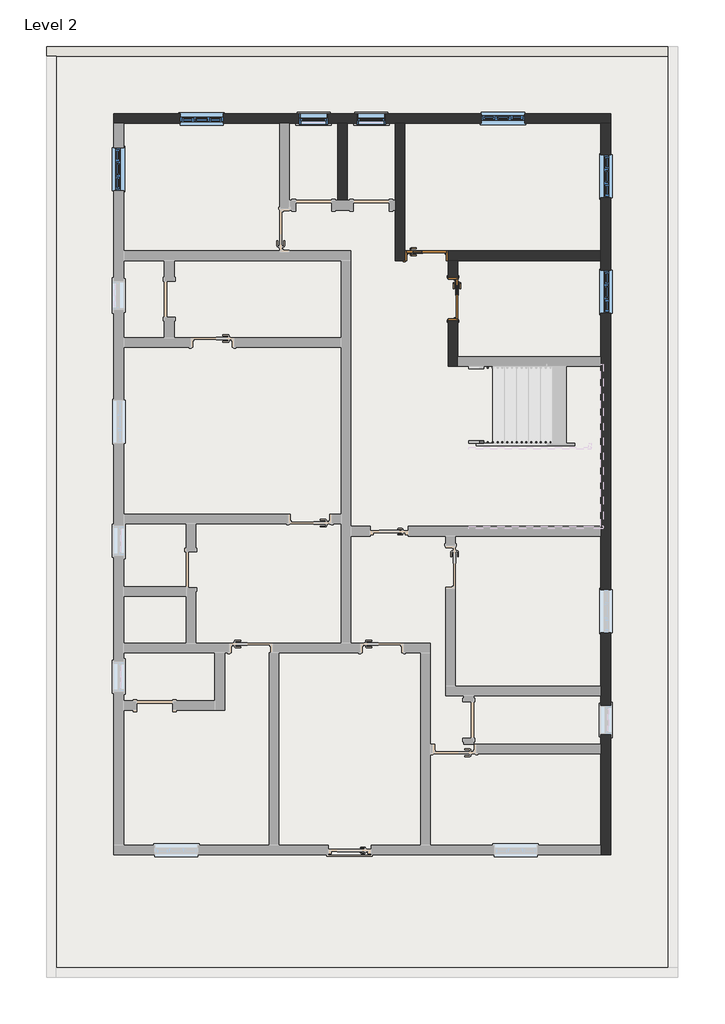
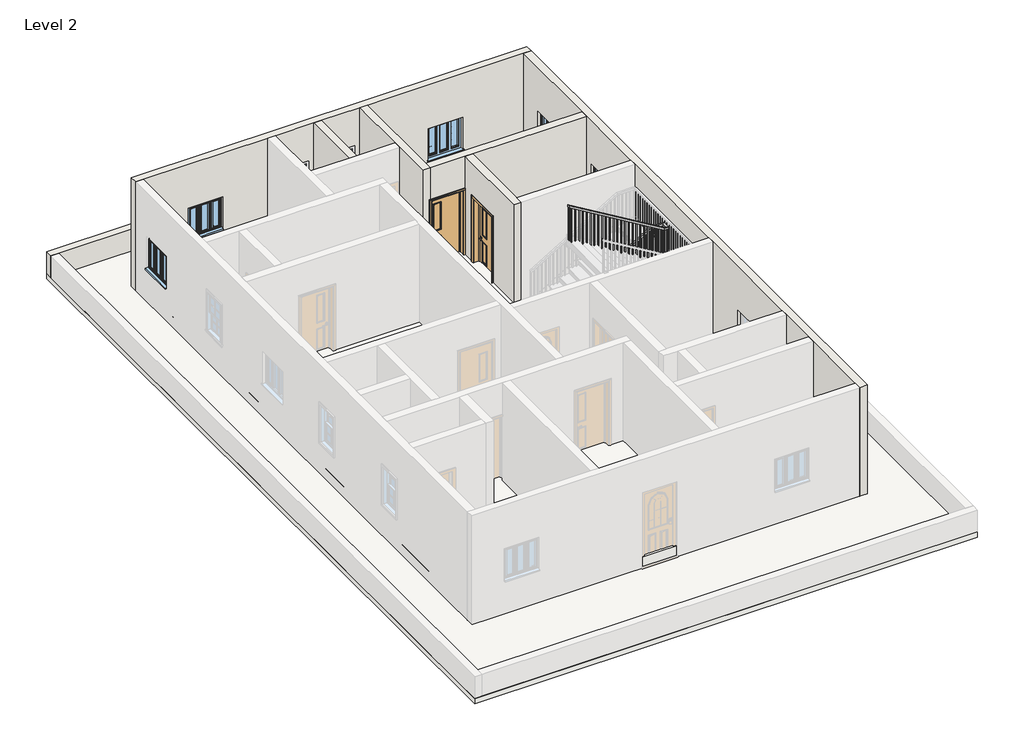
# One storey, part 2 of 3: 7 walls, 7 windows, 2 doors, 2 slabs, 1 railing, 1 roof.
"""IFC4 building model written with IfcOpenShell, lengths in millimetres."""

from ifc_helpers import new_model, si_unit, frame, origin, place, context, project, spatial, polyline, outline, extrude, faceted_brep, transform, mapped, element, save
from components import door_aa1d4bf3, window_679d2811, windows_tpl_w_glazing_bars_910x910mm_9d987a72

model = new_model("IFC4")

# Units and contexts
model_context = context("Model", 3, world=origin())
ifc_project = project(units=[si_unit("LENGTHUNIT", "METRE", prefix="MILLI")], contexts=[model_context])

# Site, building, storey
site = spatial("IfcSite", under=ifc_project)
building = spatial("IfcBuilding", under=site)
storey = spatial("IfcBuildingStorey", under=building, Name="Level 2", Elevation=3048.0)

# Doors
placement = place(None, origin())
door_shape = door_aa1d4bf3(model_context)
element("IfcDoor", 1, ObjectType="Doors_IntSgl_3 : 7'-3\"", at=placement, inside=storey, context=model_context, shape_type="MappedRepresentation", body=[
    mapped(door_shape, transform((-7303.1711241, 14069.3344295, 3048.0), x_axis=(1.0, 0.0, 0.0), y_axis=(0.0, 1.0, 0.0), z_axis=(0.0, 0.0, 1.0))),
])
element("IfcDoor", 2, ObjectType="Doors_IntSgl_3 : 7'-3\"", at=placement, inside=storey, context=model_context, shape_type="MappedRepresentation", body=[
    mapped(door_shape, transform((-6744.3711241, 13154.9344295, 3048.0), x_axis=(0.0, -1.0, 0.0), y_axis=(1.0, 0.0, 0.0), z_axis=(0.0, 0.0, 1.0))),
])

# Railing
element("IfcRailing", 3, ObjectType="Handrail - Rectangular", at=placement, inside=storey, context=model_context, shape_type="SolidModel", body=[
    faceted_brep([(-6414.1711241, 10157.7344295, 4114.8), (-6414.1711241, 10157.7344295, 4055.5575287), (-6414.1711241, 10106.9344295, 4055.5575287), (-6414.1711241, 10106.9344295, 4114.8), (-4128.1711241, 10157.7344295, 5486.4), (-4114.1003386, 10157.7344295, 5435.6), (-4114.1003386, 10106.9344295, 5435.6), (-4128.1711241, 10106.9344295, 5486.4), (-3772.5711241, 10157.7344295, 5486.4), (-3772.5711241, 10157.7344295, 5435.6), (-3823.3711241, 10106.9344295, 5435.6), (-3823.3711241, 10106.9344295, 5486.4), (-3772.5711241, 9929.1344295, 5486.4), (-3772.5711241, 9929.1344295, 5435.6), (-3823.3711241, 9979.9344295, 5435.6), (-3823.3711241, 9979.9344295, 5486.4), (-3874.1711241, 9929.1344295, 5486.4), (-3888.2419095, 9929.1344295, 5435.6), (-3888.2419095, 9979.9344295, 5435.6), (-3874.1711241, 9979.9344295, 5486.4), (-6414.1711241, 9929.1344295, 7010.4), (-6414.1711241, 9979.9344295, 7010.4), (-6414.1711241, 9979.9344295, 6951.1575287), (-6414.1711241, 9929.1344295, 6951.1575287)], [[[0, 1, 2, 3]], [[1, 0, 4, 5]], [[2, 1, 5, 6]], [[3, 2, 6, 7]], [[0, 3, 7, 4]], [[5, 4, 8, 9]], [[6, 5, 9, 10]], [[7, 6, 10, 11]], [[4, 7, 11, 8]], [[9, 8, 12, 13]], [[10, 9, 13, 14]], [[11, 10, 14, 15]], [[8, 11, 15, 12]], [[13, 12, 16, 17]], [[14, 13, 17, 18]], [[15, 14, 18, 19]], [[12, 15, 19, 16]], [[20, 21, 22, 23]], [[17, 16, 20, 23]], [[18, 17, 23, 22]], [[19, 18, 22, 21]], [[16, 19, 21, 20]]]),
    extrude(outline(polyline([(6899.7225287, -6328.4461241), (6911.1525287, -6347.4961241), (5943.6, -6347.4961241), (5943.6, -6328.4461241), (6899.7225287, -6328.4461241)])), frame((0.0, 9945.0094295, 0.0), z_axis=(0.0, 1.0, 0.0), x_axis=(0.0, 0.0, 1.0)), (0.0, 0.0, 1.0), 19.05),
    extrude(outline(polyline([(6838.7625287, -6226.8461241), (6850.1925287, -6245.8961241), (5943.6, -6245.8961241), (5943.6, -6226.8461241), (6838.7625287, -6226.8461241)])), frame((0.0, 9945.0094295, 0.0), z_axis=(0.0, 1.0, 0.0), x_axis=(0.0, 0.0, 1.0)), (0.0, 0.0, 1.0), 19.05),
    extrude(outline(polyline([(6777.8025287, -6125.2461241), (6789.2325287, -6144.2961241), (5791.2, -6144.2961241), (5791.2, -6125.2461241), (6777.8025287, -6125.2461241)])), frame((0.0, 9945.0094295, 0.0), z_axis=(0.0, 1.0, 0.0), x_axis=(0.0, 0.0, 1.0)), (0.0, 0.0, 1.0), 19.05),
    extrude(outline(polyline([(6716.8425287, -6023.6461241), (6728.2725287, -6042.6961241), (5791.2, -6042.6961241), (5791.2, -6023.6461241), (6716.8425287, -6023.6461241)])), frame((0.0, 9945.0094295, 0.0), z_axis=(0.0, 1.0, 0.0), x_axis=(0.0, 0.0, 1.0)), (0.0, 0.0, 1.0), 19.05),
    extrude(outline(polyline([(6655.8825287, -5922.0461241), (6667.3125287, -5941.0961241), (5791.2, -5941.0961241), (5791.2, -5922.0461241), (6655.8825287, -5922.0461241)])), frame((0.0, 9945.0094295, 0.0), z_axis=(0.0, 1.0, 0.0), x_axis=(0.0, 0.0, 1.0)), (0.0, 0.0, 1.0), 19.05),
    extrude(outline(polyline([(6594.9225287, -5820.4461241), (6606.3525287, -5839.4961241), (5638.8, -5839.4961241), (5638.8, -5820.4461241), (6594.9225287, -5820.4461241)])), frame((0.0, 9945.0094295, 0.0), z_axis=(0.0, 1.0, 0.0), x_axis=(0.0, 0.0, 1.0)), (0.0, 0.0, 1.0), 19.05),
    extrude(outline(polyline([(6533.9625287, -5718.8461241), (6545.3925287, -5737.8961241), (5638.8, -5737.8961241), (5638.8, -5718.8461241), (6533.9625287, -5718.8461241)])), frame((0.0, 9945.0094295, 0.0), z_axis=(0.0, 1.0, 0.0), x_axis=(0.0, 0.0, 1.0)), (0.0, 0.0, 1.0), 19.05),
    extrude(outline(polyline([(6473.0025287, -5617.2461241), (6484.4325287, -5636.2961241), (5486.4, -5636.2961241), (5486.4, -5617.2461241), (6473.0025287, -5617.2461241)])), frame((0.0, 9945.0094295, 0.0), z_axis=(0.0, 1.0, 0.0), x_axis=(0.0, 0.0, 1.0)), (0.0, 0.0, 1.0), 19.05),
    extrude(outline(polyline([(6412.0425287, -5515.6461241), (6423.4725287, -5534.6961241), (5486.4, -5534.6961241), (5486.4, -5515.6461241), (6412.0425287, -5515.6461241)])), frame((0.0, 9945.0094295, 0.0), z_axis=(0.0, 1.0, 0.0), x_axis=(0.0, 0.0, 1.0)), (0.0, 0.0, 1.0), 19.05),
    extrude(outline(polyline([(6351.0825287, -5414.0461241), (6362.5125287, -5433.0961241), (5486.4, -5433.0961241), (5486.4, -5414.0461241), (6351.0825287, -5414.0461241)])), frame((0.0, 9945.0094295, 0.0), z_axis=(0.0, 1.0, 0.0), x_axis=(0.0, 0.0, 1.0)), (0.0, 0.0, 1.0), 19.05),
    extrude(outline(polyline([(6290.1225287, -5312.4461241), (6301.5525287, -5331.4961241), (5334.0, -5331.4961241), (5334.0, -5312.4461241), (6290.1225287, -5312.4461241)])), frame((0.0, 9945.0094295, 0.0), z_axis=(0.0, 1.0, 0.0), x_axis=(0.0, 0.0, 1.0)), (0.0, 0.0, 1.0), 19.05),
    extrude(outline(polyline([(6229.1625287, -5210.8461241), (6240.5925287, -5229.8961241), (5334.0, -5229.8961241), (5334.0, -5210.8461241), (6229.1625287, -5210.8461241)])), frame((0.0, 9945.0094295, 0.0), z_axis=(0.0, 1.0, 0.0), x_axis=(0.0, 0.0, 1.0)), (0.0, 0.0, 1.0), 19.05),
    extrude(outline(polyline([(6168.2025287, -5109.2461241), (6179.6325287, -5128.2961241), (5181.6, -5128.2961241), (5181.6, -5109.2461241), (6168.2025287, -5109.2461241)])), frame((0.0, 9945.0094295, 0.0), z_axis=(0.0, 1.0, 0.0), x_axis=(0.0, 0.0, 1.0)), (0.0, 0.0, 1.0), 19.05),
    extrude(outline(polyline([(6107.2425287, -5007.6461241), (6118.6725287, -5026.6961241), (5181.6, -5026.6961241), (5181.6, -5007.6461241), (6107.2425287, -5007.6461241)])), frame((0.0, 9945.0094295, 0.0), z_axis=(0.0, 1.0, 0.0), x_axis=(0.0, 0.0, 1.0)), (0.0, 0.0, 1.0), 19.05),
    extrude(outline(polyline([(6046.2825287, -4906.0461241), (6057.7125287, -4925.0961241), (5181.6, -4925.0961241), (5181.6, -4906.0461241), (6046.2825287, -4906.0461241)])), frame((0.0, 9945.0094295, 0.0), z_axis=(0.0, 1.0, 0.0), x_axis=(0.0, 0.0, 1.0)), (0.0, 0.0, 1.0), 19.05),
    extrude(outline(polyline([(5985.3225287, -4804.4461241), (5996.7525287, -4823.4961241), (5029.2, -4823.4961241), (5029.2, -4804.4461241), (5985.3225287, -4804.4461241)])), frame((0.0, 9945.0094295, 0.0), z_axis=(0.0, 1.0, 0.0), x_axis=(0.0, 0.0, 1.0)), (0.0, 0.0, 1.0), 19.05),
    extrude(outline(polyline([(5924.3625287, -4702.8461241), (5935.7925287, -4721.8961241), (5029.2, -4721.8961241), (5029.2, -4702.8461241), (5924.3625287, -4702.8461241)])), frame((0.0, 9945.0094295, 0.0), z_axis=(0.0, 1.0, 0.0), x_axis=(0.0, 0.0, 1.0)), (0.0, 0.0, 1.0), 19.05),
    extrude(outline(polyline([(5863.4025287, -4601.2461241), (5874.8325287, -4620.2961241), (4876.8, -4620.2961241), (4876.8, -4601.2461241), (5863.4025287, -4601.2461241)])), frame((0.0, 9945.0094295, 0.0), z_axis=(0.0, 1.0, 0.0), x_axis=(0.0, 0.0, 1.0)), (0.0, 0.0, 1.0), 19.05),
    extrude(outline(polyline([(5802.4425287, -4499.6461241), (5813.8725287, -4518.6961241), (4876.8, -4518.6961241), (4876.8, -4499.6461241), (5802.4425287, -4499.6461241)])), frame((0.0, 9945.0094295, 0.0), z_axis=(0.0, 1.0, 0.0), x_axis=(0.0, 0.0, 1.0)), (0.0, 0.0, 1.0), 19.05),
    extrude(outline(polyline([(5741.4825287, -4398.0461241), (5752.9125287, -4417.0961241), (4876.8, -4417.0961241), (4876.8, -4398.0461241), (5741.4825287, -4398.0461241)])), frame((0.0, 9945.0094295, 0.0), z_axis=(0.0, 1.0, 0.0), x_axis=(0.0, 0.0, 1.0)), (0.0, 0.0, 1.0), 19.05),
    extrude(outline(polyline([(5680.5225287, -4296.4461241), (5691.9525287, -4315.4961241), (4724.4, -4315.4961241), (4724.4, -4296.4461241), (5680.5225287, -4296.4461241)])), frame((0.0, 9945.0094295, 0.0), z_axis=(0.0, 1.0, 0.0), x_axis=(0.0, 0.0, 1.0)), (0.0, 0.0, 1.0), 19.05),
    extrude(outline(polyline([(5619.5625287, -4194.8461241), (5630.9925287, -4213.8961241), (4724.4, -4213.8961241), (4724.4, -4194.8461241), (5619.5625287, -4194.8461241)])), frame((0.0, 9945.0094295, 0.0), z_axis=(0.0, 1.0, 0.0), x_axis=(0.0, 0.0, 1.0)), (0.0, 0.0, 1.0), 19.05),
    extrude(outline(polyline([(5558.6025287, -4093.2461241), (5570.0325287, -4112.2961241), (4572.0, -4112.2961241), (4572.0, -4093.2461241), (5558.6025287, -4093.2461241)])), frame((0.0, 9945.0094295, 0.0), z_axis=(0.0, 1.0, 0.0), x_axis=(0.0, 0.0, 1.0)), (0.0, 0.0, 1.0), 19.05),
    extrude(outline(polyline([(5497.6425287, -3991.6461241), (5509.0725287, -4010.6961241), (4572.0, -4010.6961241), (4572.0, -3991.6461241), (5497.6425287, -3991.6461241)])), frame((0.0, 9945.0094295, 0.0), z_axis=(0.0, 1.0, 0.0), x_axis=(0.0, 0.0, 1.0)), (0.0, 0.0, 1.0), 19.05),
    extrude(outline(polyline([(5436.6825287, -3890.0461241), (5448.1125287, -3909.0961241), (4572.0, -3909.0961241), (4572.0, -3890.0461241), (5436.6825287, -3890.0461241)])), frame((0.0, 9945.0094295, 0.0), z_axis=(0.0, 1.0, 0.0), x_axis=(0.0, 0.0, 1.0)), (0.0, 0.0, 1.0), 19.05),
    extrude(outline(polyline([(-3807.4961241, 10040.2594295), (-3788.4461241, 10040.2594295), (-3788.4461241, 10021.2094295), (-3807.4961241, 10021.2094295), (-3807.4961241, 10040.2594295)])), frame((0.0, 0.0, 4572.0), z_axis=(0.0, 0.0, 1.0), x_axis=(1.0, 0.0, 0.0)), (0.0, 0.0, 1.0), 863.6),
    extrude(outline(polyline([(-3883.6961241, 10122.8094295), (-3883.6961241, 10141.8594295), (-3864.6461241, 10141.8594295), (-3864.6461241, 10122.8094295), (-3883.6961241, 10122.8094295)])), frame((0.0, 0.0, 4572.0), z_axis=(0.0, 0.0, 1.0), x_axis=(1.0, 0.0, 0.0)), (0.0, 0.0, 1.0), 863.6),
    extrude(outline(polyline([(-3985.2961241, 10122.8094295), (-3985.2961241, 10141.8594295), (-3966.2461241, 10141.8594295), (-3966.2461241, 10122.8094295), (-3985.2961241, 10122.8094295)])), frame((0.0, 0.0, 4572.0), z_axis=(0.0, 0.0, 1.0), x_axis=(1.0, 0.0, 0.0)), (0.0, 0.0, 1.0), 863.6),
    extrude(outline(polyline([(-4086.8961241, 10122.8094295), (-4086.8961241, 10141.8594295), (-4067.8461241, 10141.8594295), (-4067.8461241, 10122.8094295), (-4086.8961241, 10122.8094295)])), frame((0.0, 0.0, 4572.0), z_axis=(0.0, 0.0, 1.0), x_axis=(1.0, 0.0, 0.0)), (0.0, 0.0, 1.0), 863.6),
    extrude(outline(polyline([(5402.3925287, -4169.4461241), (5390.9625287, -4188.4961241), (4419.6, -4188.4961241), (4419.6, -4169.4461241), (5402.3925287, -4169.4461241)])), frame((0.0, 10122.8094295, 0.0), z_axis=(0.0, 1.0, 0.0), x_axis=(0.0, 0.0, 1.0)), (0.0, 0.0, 1.0), 19.05),
    extrude(outline(polyline([(5341.4325287, -4271.0461241), (5330.0025287, -4290.0961241), (4419.6, -4290.0961241), (4419.6, -4271.0461241), (5341.4325287, -4271.0461241)])), frame((0.0, 10122.8094295, 0.0), z_axis=(0.0, 1.0, 0.0), x_axis=(0.0, 0.0, 1.0)), (0.0, 0.0, 1.0), 19.05),
    extrude(outline(polyline([(5280.4725287, -4372.6461241), (5269.0425287, -4391.6961241), (4419.6, -4391.6961241), (4419.6, -4372.6461241), (5280.4725287, -4372.6461241)])), frame((0.0, 10122.8094295, 0.0), z_axis=(0.0, 1.0, 0.0), x_axis=(0.0, 0.0, 1.0)), (0.0, 0.0, 1.0), 19.05),
    extrude(outline(polyline([(5219.5125287, -4474.2461241), (5208.0825287, -4493.2961241), (4267.2, -4493.2961241), (4267.2, -4474.2461241), (5219.5125287, -4474.2461241)])), frame((0.0, 10122.8094295, 0.0), z_axis=(0.0, 1.0, 0.0), x_axis=(0.0, 0.0, 1.0)), (0.0, 0.0, 1.0), 19.05),
    extrude(outline(polyline([(5158.5525287, -4575.8461241), (5147.1225287, -4594.8961241), (4267.2, -4594.8961241), (4267.2, -4575.8461241), (5158.5525287, -4575.8461241)])), frame((0.0, 10122.8094295, 0.0), z_axis=(0.0, 1.0, 0.0), x_axis=(0.0, 0.0, 1.0)), (0.0, 0.0, 1.0), 19.05),
    extrude(outline(polyline([(5097.5925287, -4677.4461241), (5086.1625287, -4696.4961241), (4114.8, -4696.4961241), (4114.8, -4677.4461241), (5097.5925287, -4677.4461241)])), frame((0.0, 10122.8094295, 0.0), z_axis=(0.0, 1.0, 0.0), x_axis=(0.0, 0.0, 1.0)), (0.0, 0.0, 1.0), 19.05),
    extrude(outline(polyline([(5036.6325287, -4779.0461241), (5025.2025287, -4798.0961241), (4114.8, -4798.0961241), (4114.8, -4779.0461241), (5036.6325287, -4779.0461241)])), frame((0.0, 10122.8094295, 0.0), z_axis=(0.0, 1.0, 0.0), x_axis=(0.0, 0.0, 1.0)), (0.0, 0.0, 1.0), 19.05),
    extrude(outline(polyline([(4975.6725287, -4880.6461241), (4964.2425287, -4899.6961241), (4114.8, -4899.6961241), (4114.8, -4880.6461241), (4975.6725287, -4880.6461241)])), frame((0.0, 10122.8094295, 0.0), z_axis=(0.0, 1.0, 0.0), x_axis=(0.0, 0.0, 1.0)), (0.0, 0.0, 1.0), 19.05),
    extrude(outline(polyline([(4914.7125287, -4982.2461241), (4903.2825287, -5001.2961241), (3962.4, -5001.2961241), (3962.4, -4982.2461241), (4914.7125287, -4982.2461241)])), frame((0.0, 10122.8094295, 0.0), z_axis=(0.0, 1.0, 0.0), x_axis=(0.0, 0.0, 1.0)), (0.0, 0.0, 1.0), 19.05),
    extrude(outline(polyline([(4853.7525287, -5083.8461241), (4842.3225287, -5102.8961241), (3962.4, -5102.8961241), (3962.4, -5083.8461241), (4853.7525287, -5083.8461241)])), frame((0.0, 10122.8094295, 0.0), z_axis=(0.0, 1.0, 0.0), x_axis=(0.0, 0.0, 1.0)), (0.0, 0.0, 1.0), 19.05),
    extrude(outline(polyline([(4792.7925287, -5185.4461241), (4781.3625287, -5204.4961241), (3810.0, -5204.4961241), (3810.0, -5185.4461241), (4792.7925287, -5185.4461241)])), frame((0.0, 10122.8094295, 0.0), z_axis=(0.0, 1.0, 0.0), x_axis=(0.0, 0.0, 1.0)), (0.0, 0.0, 1.0), 19.05),
    extrude(outline(polyline([(4731.8325287, -5287.0461241), (4720.4025287, -5306.0961241), (3810.0, -5306.0961241), (3810.0, -5287.0461241), (4731.8325287, -5287.0461241)])), frame((0.0, 10122.8094295, 0.0), z_axis=(0.0, 1.0, 0.0), x_axis=(0.0, 0.0, 1.0)), (0.0, 0.0, 1.0), 19.05),
    extrude(outline(polyline([(4670.8725287, -5388.6461241), (4659.4425287, -5407.6961241), (3810.0, -5407.6961241), (3810.0, -5388.6461241), (4670.8725287, -5388.6461241)])), frame((0.0, 10122.8094295, 0.0), z_axis=(0.0, 1.0, 0.0), x_axis=(0.0, 0.0, 1.0)), (0.0, 0.0, 1.0), 19.05),
    extrude(outline(polyline([(4609.9125287, -5490.2461241), (4598.4825287, -5509.2961241), (3657.6, -5509.2961241), (3657.6, -5490.2461241), (4609.9125287, -5490.2461241)])), frame((0.0, 10122.8094295, 0.0), z_axis=(0.0, 1.0, 0.0), x_axis=(0.0, 0.0, 1.0)), (0.0, 0.0, 1.0), 19.05),
    extrude(outline(polyline([(4548.9525287, -5591.8461241), (4537.5225287, -5610.8961241), (3657.6, -5610.8961241), (3657.6, -5591.8461241), (4548.9525287, -5591.8461241)])), frame((0.0, 10122.8094295, 0.0), z_axis=(0.0, 1.0, 0.0), x_axis=(0.0, 0.0, 1.0)), (0.0, 0.0, 1.0), 19.05),
    extrude(outline(polyline([(4487.9925287, -5693.4461241), (4476.5625287, -5712.4961241), (3505.2, -5712.4961241), (3505.2, -5693.4461241), (4487.9925287, -5693.4461241)])), frame((0.0, 10122.8094295, 0.0), z_axis=(0.0, 1.0, 0.0), x_axis=(0.0, 0.0, 1.0)), (0.0, 0.0, 1.0), 19.05),
    extrude(outline(polyline([(4427.0325287, -5795.0461241), (4415.6025287, -5814.0961241), (3505.2, -5814.0961241), (3505.2, -5795.0461241), (4427.0325287, -5795.0461241)])), frame((0.0, 10122.8094295, 0.0), z_axis=(0.0, 1.0, 0.0), x_axis=(0.0, 0.0, 1.0)), (0.0, 0.0, 1.0), 19.05),
    extrude(outline(polyline([(4366.0725287, -5896.6461241), (4354.6425287, -5915.6961241), (3505.2, -5915.6961241), (3505.2, -5896.6461241), (4366.0725287, -5896.6461241)])), frame((0.0, 10122.8094295, 0.0), z_axis=(0.0, 1.0, 0.0), x_axis=(0.0, 0.0, 1.0)), (0.0, 0.0, 1.0), 19.05),
    extrude(outline(polyline([(4305.1125287, -5998.2461241), (4293.6825287, -6017.2961241), (3352.8, -6017.2961241), (3352.8, -5998.2461241), (4305.1125287, -5998.2461241)])), frame((0.0, 10122.8094295, 0.0), z_axis=(0.0, 1.0, 0.0), x_axis=(0.0, 0.0, 1.0)), (0.0, 0.0, 1.0), 19.05),
    extrude(outline(polyline([(4244.1525287, -6099.8461241), (4232.7225287, -6118.8961241), (3352.8, -6118.8961241), (3352.8, -6099.8461241), (4244.1525287, -6099.8461241)])), frame((0.0, 10122.8094295, 0.0), z_axis=(0.0, 1.0, 0.0), x_axis=(0.0, 0.0, 1.0)), (0.0, 0.0, 1.0), 19.05),
    extrude(outline(polyline([(4183.1925287, -6201.4461241), (4171.7625287, -6220.4961241), (3200.4, -6220.4961241), (3200.4, -6201.4461241), (4183.1925287, -6201.4461241)])), frame((0.0, 10122.8094295, 0.0), z_axis=(0.0, 1.0, 0.0), x_axis=(0.0, 0.0, 1.0)), (0.0, 0.0, 1.0), 19.05),
    extrude(outline(polyline([(4122.2325287, -6303.0461241), (4110.8025287, -6322.0961241), (3200.4, -6322.0961241), (3200.4, -6303.0461241), (4122.2325287, -6303.0461241)])), frame((0.0, 10122.8094295, 0.0), z_axis=(0.0, 1.0, 0.0), x_axis=(0.0, 0.0, 1.0)), (0.0, 0.0, 1.0), 19.05),
    extrude(outline(polyline([(-3807.4961241, 9964.0594295), (-3788.4461241, 9964.0594295), (-3788.4461241, 9945.0094295), (-3807.4961241, 9945.0094295), (-3807.4961241, 9964.0594295)])), frame((0.0, 0.0, 4572.0), z_axis=(0.0, 0.0, 1.0), x_axis=(1.0, 0.0, 0.0)), (0.0, 0.0, 1.0), 863.6),
    extrude(outline(polyline([(-3807.4961241, 10122.8094295), (-3807.4961241, 10141.8594295), (-3788.4461241, 10141.8594295), (-3788.4461241, 10122.8094295), (-3807.4961241, 10122.8094295)])), frame((0.0, 0.0, 4572.0), z_axis=(0.0, 0.0, 1.0), x_axis=(1.0, 0.0, 0.0)), (0.0, 0.0, 1.0), 863.6),
    extrude(outline(polyline([(6939.7275287, -6395.1211241), (6951.1575287, -6414.1711241), (5943.6, -6414.1711241), (5943.6, -6395.1211241), (6939.7275287, -6395.1211241)])), frame((0.0, 9945.0094295, 0.0), z_axis=(0.0, 1.0, 0.0), x_axis=(0.0, 0.0, 1.0)), (0.0, 0.0, 1.0), 19.05),
    extrude(outline(polyline([(4066.9875287, -6395.1211241), (4055.5575287, -6414.1711241), (3200.4, -6414.1711241), (3200.4, -6395.1211241), (4066.9875287, -6395.1211241)])), frame((0.0, 10122.8094295, 0.0), z_axis=(0.0, 1.0, 0.0), x_axis=(0.0, 0.0, 1.0)), (0.0, 0.0, 1.0), 19.05),
])

# Roof
element("IfcRoof", 4, ObjectType="Generic - 12\"", at=placement, inside=storey, context=model_context, shape_type="SweptSolid", body=[
    extrude(outline(polyline([(-13907.1711241, 17066.5344295), (-3416.9711241, 17066.5344295), (-3416.9711241, 1420.1344295), (-13907.1711241, 1420.1344295), (-13907.1711241, 17066.5344295)])), frame((0.0, 0.0, 3048.0), z_axis=(0.0, 0.0, 1.0), x_axis=(1.0, 0.0, 0.0)), (0.0, 0.0, 1.0), 304.8),
])

# Slabs
element("IfcSlab", 5, ObjectType="Generic - 12\" 2", at=placement, inside=storey, context=model_context, shape_type="SweptSolid", body=[
    extrude(outline(polyline([(-3416.9711241, 17066.5344295), (-3416.9711241, 1420.1344295), (-13907.1711241, 1420.1344295), (-13907.1711241, 17066.5344295), (-3416.9711241, 17066.5344295)])), frame((0.0, 0.0, 2895.6), z_axis=(0.0, 0.0, 1.0), x_axis=(1.0, 0.0, 0.0)), (0.0, 0.0, 1.0), 152.4),
])
element("IfcSlab", 6, ObjectType="Generic - 12\" 3", at=placement, inside=storey, context=model_context, shape_type="SweptSolid", body=[
    extrude(outline(polyline([(-1994.5711241, 18488.2009778), (-1994.5711241, -1171.3990222), (-15329.5711241, -1171.3990222), (-15329.5711241, 18488.2009778), (-1994.5711241, 18488.2009778)])), frame((0.0, 0.0, 2895.6), z_axis=(0.0, 0.0, 1.0), x_axis=(1.0, 0.0, 0.0)), (0.0, 0.0, 1.0), 152.4),
])

# Walls
element("IfcWall", 7, ObjectType="Generic -4.5\" p", at=placement, inside=storey, context=model_context, shape_type="SweptSolid", body=[
    extrude(outline(polyline([(-9182.7711241, 15237.7344295), (-9182.7711241, 16863.3344295), (-8979.5711241, 16863.3344295), (-8979.5711241, 15237.7344295), (-9182.7711241, 15237.7344295)])), frame((0.0, 0.0, 3048.0), z_axis=(0.0, 0.0, 1.0), x_axis=(1.0, 0.0, 0.0)), (0.0, 0.0, 1.0), 3048.0),
])
element("IfcWall", 8, ObjectType="Generic -4.5\" p", at=placement, inside=storey, context=model_context, shape_type="Brep", body=[
    faceted_brep([(-7963.5711241, 16863.3344295, 3048.0), (-7963.5711241, 15237.7344295, 3048.0), (-7963.5711241, 15034.5344295, 3048.0), (-7963.5711241, 13967.7344295, 3048.0), (-7963.5711241, 13967.7344295, 6096.0), (-7963.5711241, 15034.5344295, 6096.0), (-7963.5711241, 15237.7344295, 6096.0), (-7963.5711241, 16863.3344295, 6096.0), (-7760.3711241, 16863.3344295, 3048.0), (-7760.3711241, 16863.3344295, 6096.0), (-7760.3711241, 14170.9344295, 6096.0), (-7760.3711241, 13967.7344295, 6096.0), (-7760.3711241, 13967.7344295, 5181.6), (-7760.3711241, 13967.7344295, 3048.0)], [[[0, 1, 2, 3, 4, 5, 6, 7]], [[8, 9, 10, 11, 12, 13]], [[3, 2, 1, 0, 8, 13]], [[7, 6, 5, 4, 11, 10, 9]], [[0, 7, 9, 8]], [[4, 3, 13, 12, 11]]]),
])
element("IfcWall", 9, ObjectType="Generic -4.5\" p", at=placement, inside=storey, context=model_context, shape_type="Brep", body=[
    faceted_brep([(-7760.3711241, 14170.9344295, 6096.0), (-3620.1711241, 14170.9344295, 6096.0), (-3620.1711241, 14170.9344295, 3048.0), (-6845.9711241, 14170.9344295, 3048.0), (-6845.9711241, 14170.9344295, 5181.6), (-7760.3711241, 14170.9344295, 5181.6), (-3620.1711241, 13967.7344295, 6096.0), (-6642.7711241, 13967.7344295, 6096.0), (-6845.9711241, 13967.7344295, 6096.0), (-7760.3711241, 13967.7344295, 6096.0), (-7760.3711241, 13967.7344295, 5181.6), (-6845.9711241, 13967.7344295, 5181.6), (-6845.9711241, 13967.7344295, 3048.0), (-6642.7711241, 13967.7344295, 3048.0), (-3620.1711241, 13967.7344295, 3048.0)], [[[0, 1, 2, 3, 4, 5]], [[6, 7, 8, 9, 10, 11, 12, 13, 14]], [[2, 14, 13, 12, 3]], [[1, 0, 9, 8, 7, 6]], [[9, 0, 5, 10]], [[2, 1, 6, 14]], [[11, 4, 3, 12]], [[4, 11, 10, 5]]]),
])
element("IfcWall", 10, ObjectType="Generic -4.5\" p", at=placement, inside=storey, context=model_context, shape_type="Brep", body=[
    faceted_brep([(-6845.9711241, 11732.5344295, 6096.0), (-6845.9711241, 13967.7344295, 6096.0), (-6845.9711241, 13967.7344295, 5181.6), (-6845.9711241, 13967.7344295, 3048.0), (-6845.9711241, 13612.1344295, 3048.0), (-6845.9711241, 13612.1344295, 5181.6), (-6845.9711241, 12697.7344295, 5181.6), (-6845.9711241, 12697.7344295, 3048.0), (-6845.9711241, 11732.5344295, 3048.0), (-6642.7711241, 13967.7344295, 6096.0), (-6642.7711241, 11935.7344295, 6096.0), (-6642.7711241, 11732.5344295, 6096.0), (-6642.7711241, 11732.5344295, 3048.0), (-6642.7711241, 11935.7344295, 3048.0), (-6642.7711241, 12697.7344295, 3048.0), (-6642.7711241, 12697.7344295, 5181.6), (-6642.7711241, 13612.1344295, 5181.6), (-6642.7711241, 13612.1344295, 3048.0), (-6642.7711241, 13967.7344295, 3048.0)], [[[0, 1, 2, 3, 4, 5, 6, 7, 8]], [[9, 10, 11, 12, 13, 14, 15, 16, 17, 18]], [[3, 18, 17, 4]], [[12, 8, 7, 14, 13]], [[1, 0, 11, 10, 9]], [[3, 2, 1, 9, 18]], [[0, 8, 12, 11]], [[6, 15, 14, 7]], [[15, 6, 5, 16]], [[16, 5, 4, 17]]]),
])
element("IfcWall", 11, ObjectType="Generic -4.5\" p", at=placement, inside=storey, context=model_context, shape_type="Brep", body=[
    faceted_brep([(-15329.5711241, 18285.0009778, 3048.0), (-15126.3711241, 18285.0009778, 3048.0), (-2197.7711241, 18285.0009778, 3048.0), (-2197.7711241, 18285.0009778, 3657.6), (-15126.3711241, 18285.0009778, 3657.6), (-15329.5711241, 18285.0009778, 3657.6), (-15329.5711241, 18488.2009778, 3048.0), (-15329.5711241, 18488.2009778, 3657.6), (-2197.7711241, 18488.2009778, 3657.6), (-2197.7711241, 18488.2009778, 3048.0)], [[[0, 1, 2, 3, 4, 5]], [[6, 7, 8, 9]], [[2, 1, 0, 6, 9]], [[5, 4, 3, 8, 7]], [[0, 5, 7, 6]], [[3, 2, 9, 8]]]),
])
element("IfcWall", 12, ObjectType="Generic -9\" w", at=placement, inside=storey, context=model_context, shape_type="Brep", body=[
    faceted_brep([(-13907.1711241, 16863.3344295, 3048.0), (-13703.9711241, 16863.3344295, 3048.0), (-10401.9711241, 16863.3344295, 3048.0), (-10198.7711241, 16863.3344295, 3048.0), (-9182.7711241, 16863.3344295, 3048.0), (-8979.5711241, 16863.3344295, 3048.0), (-7963.5711241, 16863.3344295, 3048.0), (-7760.3711241, 16863.3344295, 3048.0), (-3620.1711241, 16863.3344295, 3048.0), (-3416.9711241, 16863.3344295, 3048.0), (-3416.9711241, 16863.3344295, 6096.0), (-3620.1711241, 16863.3344295, 6096.0), (-7760.3711241, 16863.3344295, 6096.0), (-7963.5711241, 16863.3344295, 6096.0), (-8979.5711241, 16863.3344295, 6096.0), (-9182.7711241, 16863.3344295, 6096.0), (-10198.7711241, 16863.3344295, 6096.0), (-10401.9711241, 16863.3344295, 6096.0), (-13703.9711241, 16863.3344295, 6096.0), (-13907.1711241, 16863.3344295, 6096.0), (-11597.9711241, 16863.3344295, 4872.4), (-11597.9711241, 16863.3344295, 3962.4), (-12507.9711241, 16863.3344295, 3962.4), (-12507.9711241, 16863.3344295, 4872.4), (-6145.2711241, 16863.3344295, 4872.4), (-5235.2711241, 16863.3344295, 4872.4), (-5235.2711241, 16863.3344295, 3962.4), (-6145.2711241, 16863.3344295, 3962.4), (-9385.9711241, 16863.3344295, 5029.2), (-9385.9711241, 16863.3344295, 3962.4), (-9995.5711241, 16863.3344295, 3962.4), (-9995.5711241, 16863.3344295, 5029.2), (-8166.7711241, 16863.3344295, 5029.2), (-8166.7711241, 16863.3344295, 3962.4), (-8776.3711241, 16863.3344295, 3962.4), (-8776.3711241, 16863.3344295, 5029.2), (-13907.1711241, 17066.5344295, 3048.0), (-13907.1711241, 17066.5344295, 6096.0), (-3416.9711241, 17066.5344295, 6096.0), (-3416.9711241, 17066.5344295, 3048.0), (-11597.9711241, 17066.5344295, 4872.4), (-12507.9711241, 17066.5344295, 4872.4), (-12507.9711241, 17066.5344295, 3962.4), (-11597.9711241, 17066.5344295, 3962.4), (-6145.2711241, 17066.5344295, 4872.4), (-6145.2711241, 17066.5344295, 3962.4), (-5235.2711241, 17066.5344295, 3962.4), (-5235.2711241, 17066.5344295, 4872.4), (-9385.9711241, 17066.5344295, 5029.2), (-9995.5711241, 17066.5344295, 5029.2), (-9995.5711241, 17066.5344295, 3962.4), (-9385.9711241, 17066.5344295, 3962.4), (-8166.7711241, 17066.5344295, 5029.2), (-8776.3711241, 17066.5344295, 5029.2), (-8776.3711241, 17066.5344295, 3962.4), (-8166.7711241, 17066.5344295, 3962.4)], [[[0, 1, 2, 3, 4, 5, 6, 7, 8, 9, 10, 11, 12, 13, 14, 15, 16, 17, 18, 19], [20, 21, 22, 23], [24, 25, 26, 27], [28, 29, 30, 31], [32, 33, 34, 35]], [[36, 37, 38, 39], [40, 41, 42, 43], [44, 45, 46, 47], [48, 49, 50, 51], [52, 53, 54, 55]], [[9, 8, 7, 6, 5, 4, 3, 2, 1, 0, 36, 39]], [[19, 18, 17, 16, 15, 14, 13, 12, 11, 10, 38, 37]], [[10, 9, 39, 38]], [[0, 19, 37, 36]], [[21, 20, 40, 43]], [[22, 21, 43, 42]], [[23, 22, 42, 41]], [[20, 23, 41, 40]], [[45, 44, 24, 27]], [[46, 45, 27, 26]], [[47, 46, 26, 25]], [[44, 47, 25, 24]], [[29, 28, 48, 51]], [[30, 29, 51, 50]], [[31, 30, 50, 49]], [[28, 31, 49, 48]], [[33, 32, 52, 55]], [[34, 33, 55, 54]], [[35, 34, 54, 53]], [[32, 35, 53, 52]]]),
])
element("IfcWall", 13, ObjectType="Generic -9\" w", at=placement, inside=storey, context=model_context, shape_type="Brep", body=[
    faceted_brep([(-3620.1711241, 16863.3344295, 3048.0), (-3620.1711241, 14170.9344295, 3048.0), (-3620.1711241, 13967.7344295, 3048.0), (-3620.1711241, 11935.7344295, 3048.0), (-3620.1711241, 11732.5344295, 3048.0), (-3620.1711241, 8354.3344295, 3048.0), (-3620.1711241, 8151.1344295, 3048.0), (-3620.1711241, 4976.1344295, 3048.0), (-3620.1711241, 4772.9344295, 3048.0), (-3620.1711241, 3756.9344295, 3048.0), (-3620.1711241, 3553.7344295, 3048.0), (-3620.1711241, 1623.3344295, 3048.0), (-3620.1711241, 1420.1344295, 3048.0), (-3620.1711241, 1420.1344295, 6096.0), (-3620.1711241, 1623.3344295, 6096.0), (-3620.1711241, 3553.7344295, 6096.0), (-3620.1711241, 3756.9344295, 6096.0), (-3620.1711241, 4772.9344295, 6096.0), (-3620.1711241, 4976.1344295, 6096.0), (-3620.1711241, 8151.1344295, 6096.0), (-3620.1711241, 8354.3344295, 6096.0), (-3620.1711241, 11732.5344295, 6096.0), (-3620.1711241, 11935.7344295, 6096.0), (-3620.1711241, 13967.7344295, 6096.0), (-3620.1711241, 14170.9344295, 6096.0), (-3620.1711241, 16863.3344295, 6096.0), (-3620.1711241, 16200.7344295, 4872.4), (-3620.1711241, 15290.7344295, 4872.4), (-3620.1711241, 15290.7344295, 3962.4), (-3620.1711241, 16200.7344295, 3962.4), (-3620.1711241, 13762.3344295, 4872.4), (-3620.1711241, 12852.3344295, 4872.4), (-3620.1711241, 12852.3344295, 3962.4), (-3620.1711241, 13762.3344295, 3962.4), (-3620.1711241, 7018.6344295, 4872.4), (-3620.1711241, 6108.6344295, 4872.4), (-3620.1711241, 6108.6344295, 3962.4), (-3620.1711241, 7018.6344295, 3962.4), (-3620.1711241, 4569.7344295, 5029.2), (-3620.1711241, 3960.1344295, 5029.2), (-3620.1711241, 3960.1344295, 3962.4), (-3620.1711241, 4569.7344295, 3962.4), (-3416.9711241, 16863.3344295, 3048.0), (-3416.9711241, 16863.3344295, 6096.0), (-3416.9711241, 1420.1344295, 6096.0), (-3416.9711241, 1420.1344295, 3048.0), (-3416.9711241, 16200.7344295, 4872.4), (-3416.9711241, 16200.7344295, 3962.4), (-3416.9711241, 15290.7344295, 3962.4), (-3416.9711241, 15290.7344295, 4872.4), (-3416.9711241, 13762.3344295, 4872.4), (-3416.9711241, 13762.3344295, 3962.4), (-3416.9711241, 12852.3344295, 3962.4), (-3416.9711241, 12852.3344295, 4872.4), (-3416.9711241, 7018.6344295, 4872.4), (-3416.9711241, 7018.6344295, 3962.4), (-3416.9711241, 6108.6344295, 3962.4), (-3416.9711241, 6108.6344295, 4872.4), (-3416.9711241, 4569.7344295, 5029.2), (-3416.9711241, 4569.7344295, 3962.4), (-3416.9711241, 3960.1344295, 3962.4), (-3416.9711241, 3960.1344295, 5029.2)], [[[0, 1, 2, 3, 4, 5, 6, 7, 8, 9, 10, 11, 12, 13, 14, 15, 16, 17, 18, 19, 20, 21, 22, 23, 24, 25], [26, 27, 28, 29], [30, 31, 32, 33], [34, 35, 36, 37], [38, 39, 40, 41]], [[42, 43, 44, 45], [46, 47, 48, 49], [50, 51, 52, 53], [54, 55, 56, 57], [58, 59, 60, 61]], [[12, 11, 10, 9, 8, 7, 6, 5, 4, 3, 2, 1, 0, 42, 45]], [[25, 24, 23, 22, 21, 20, 19, 18, 17, 16, 15, 14, 13, 44, 43]], [[0, 25, 43, 42]], [[13, 12, 45, 44]], [[47, 46, 26, 29]], [[48, 47, 29, 28]], [[49, 48, 28, 27]], [[46, 49, 27, 26]], [[51, 50, 30, 33]], [[52, 51, 33, 32]], [[53, 52, 32, 31]], [[50, 53, 31, 30]], [[55, 54, 34, 37]], [[56, 55, 37, 36]], [[57, 56, 36, 35]], [[54, 57, 35, 34]], [[59, 58, 38, 41]], [[60, 59, 41, 40]], [[61, 60, 40, 39]], [[58, 61, 39, 38]]]),
])

# Windows
window_shape = window_679d2811(model_context)
element("IfcWindow", 14, ObjectType="Window-Double-Hung : 24\" x 42\"", at=placement, inside=storey, context=model_context, shape_type="MappedRepresentation", body=[
    mapped(window_shape, transform((-9690.7711241, 16964.9344295, 3048.0), x_axis=(-1.0, 0.0, 0.0), y_axis=(0.0, -1.0, 0.0), z_axis=(0.0, 0.0, 1.0))),
])
element("IfcWindow", 15, ObjectType="Window-Double-Hung : 24\" x 42\"", at=placement, inside=storey, context=model_context, shape_type="MappedRepresentation", body=[
    mapped(window_shape, transform((-8471.5711241, 16964.9344295, 3048.0), x_axis=(-1.0, 0.0, 0.0), y_axis=(0.0, -1.0, 0.0), z_axis=(0.0, 0.0, 1.0))),
])
windows_tpl_w_glazing_bars_910x910mm_shape = windows_tpl_w_glazing_bars_910x910mm_9d987a72(model_context)
element("IfcWindow", 16, ObjectType="Windows_Tpl_w-Glazing_Bars : 910x910mm", at=placement, inside=storey, context=model_context, shape_type="MappedRepresentation", body=[
    mapped(windows_tpl_w_glazing_bars_910x910mm_shape, transform((-12289.6377907, 16973.3909974, 2762.4), x_axis=(-1.0, 0.0, 0.0), y_axis=(0.0, -1.0, 0.0), z_axis=(0.0, 0.0, 1.0))),
])
element("IfcWindow", 17, ObjectType="Windows_Tpl_w-Glazing_Bars : 910x910mm", at=placement, inside=storey, context=model_context, shape_type="MappedRepresentation", body=[
    mapped(windows_tpl_w_glazing_bars_910x910mm_shape, transform((-5453.6044574, 16956.4778617, 2762.4), x_axis=(1.0, 0.0, 0.0), y_axis=(0.0, 1.0, 0.0), z_axis=(0.0, 0.0, 1.0))),
])
element("IfcWindow", 18, ObjectType="Windows_Tpl_w-Glazing_Bars : 910x910mm", at=placement, inside=storey, context=model_context, shape_type="MappedRepresentation", body=[
    mapped(windows_tpl_w_glazing_bars_910x910mm_shape, transform((-3527.0276919, 15509.0677629, 2762.4), x_axis=(0.0, -1.0, 0.0), y_axis=(1.0, 0.0, 0.0), z_axis=(0.0, 0.0, 1.0))),
])
element("IfcWindow", 19, ObjectType="Windows_Tpl_w-Glazing_Bars : 910x910mm", at=placement, inside=storey, context=model_context, shape_type="MappedRepresentation", body=[
    mapped(windows_tpl_w_glazing_bars_910x910mm_shape, transform((-13797.1145562, 16134.8010962, 2762.4), x_axis=(0.0, 1.0, 0.0), y_axis=(-1.0, 0.0, 0.0), z_axis=(0.0, 0.0, 1.0))),
])
element("IfcWindow", 20, ObjectType="Windows_Tpl_w-Glazing_Bars : 910x910mm", at=placement, inside=storey, context=model_context, shape_type="MappedRepresentation", body=[
    mapped(windows_tpl_w_glazing_bars_910x910mm_shape, transform((-3527.0276919, 13070.6677629, 2762.4), x_axis=(0.0, -1.0, 0.0), y_axis=(1.0, 0.0, 0.0), z_axis=(0.0, 0.0, 1.0))),
])

save(model, "model.ifc")

# Revit data of these elements
# Type "Doors_IntSgl_3 : 7'-3\""
#   Type Mark = "14"
#   Type Comments = "Internal Single"
#   Operation = "SingleSwingRight"
#   Construction Type Id = "SGL"
#   Manufacturer = "Revit"
#   Keynote = "L20"
#   Description = "Internal Single Door"
#   Analytic Construction = "Large single-glazed windows"
#   Visual Light Transmittance = 0.9
#   VisionPanel Width = 0' - 7.87402"
#   UnderCut = 0' - 0.31496"
#   Tolerance = 0' - 0.07874"
#   Structural Tolerance = 0' - 0.31496"
#   StopDepth = 0' - 1.25984"
#   Stop Thickness = 0' - 0.74803"
#   Stile Top of Lock Rail = 3' - 7.30709"
#   Stile Top Rail = 0' - 8.85827"
#   Stile Shutting = 0' - 4.92126"
#   Stile Lock Rail = 0' - 6.88976"
#   Stile Bottom Rail = 1' - 1.77953"
#   Solar Heat Gain Coefficient = 0.86
#   Rough Width = 3' - 0"
#   Rough Height = 7' - 0"
#   Heat Transfer Coefficient (U) = 0.979472 BTU/(h·ft²·°F)
#   Handle Z Distance = 3' - 3.37008"
#   Handle X Distance = 0' - 2.95276"
#   Frame Thickness = 0' - 1.25984"
#   Door Panel Width = 2' - 8.69291"
#   Door Panel Thickness = 0' - 1.49606"
#   Door Panel Offset = 0' - 0"
#   Height = 7' - 0"
#   Width = 3' - 0"
#   Door Panel Height = 6' - 10.0315"
#   Architrave Setback = 0' - 0.19685"
#   Vis - Ironmongery = yes
#   Define Thermal Properties by = 1
#   Material Ironmongery = Door - Handle
#   Material Glass = Door - Glazing
#   Material Frame = Door - Frame/Mullion
#   Material Door = Door - Panel
#   Material Beading = Door - Panel
#   Material Architrave = Door - Architrave
#   Function = (empty or 0)
#   Wall Closure = (empty or 0)
# Type "Handrail - Rectangular"
#   Assembly Code = "C2010400"
#   built-in parameter 1008612 = 0.0416667 (stored number, unit not read)
#   built-in parameter 1008611 = 0.0416667 (stored number, unit not read)
#   built-in parameter 1008609 = 0.333333 (stored number, unit not read)
#   built-in parameter 1008604 = 0.166667 (stored number, unit not read)
#   built-in parameter 1008603 = 0.166667 (stored number, unit not read)
#   Railing Height = 3' - 0"
#   built-in parameter 1008630 = 2
#   built-in parameter 1008610 = 2
#   built-in parameter 1008618 = Baluster - Square : 3/4"
# Type "Generic - 12\""
#   Assembly Code = "B1020"
#   Layers, outside or top first: 1' - 0" no material (function 1)
# Type "Generic - 12\" 2"
#   Assembly Code = "B1010"
#   Function = 0
#   Layers, outside or top first: 0' - 6" no material (function 1)
# Type "Generic - 12\" 3"
#   Assembly Code = "B1010"
#   Function = 0
#   Layers, outside or top first: 0' - 6" no material (function 1)
# Type "Generic -4.5\" p"
#   Assembly Code = "B2010"
#   Layers, outside or top first: 0' - 8" no material (function 1)
# Type "Generic -9\" w"
#   Assembly Code = "B2010"
#   Layers, outside or top first: 0' - 8" no material (function 1)
# Type "Window-Double-Hung : 24\" x 42\""
#   Type Mark = "10"
#   Fire Rating = "0.5h"
#   Construction Type Id = "DG-DR"
#   Assembly Code = "B2020100"
#   Analytic Construction = "Double glazing - domestic"
#   Wall Thickness [instance default] = 0' - 6"
#   Window Inset [instance default] = 0' - 0"
#   Visual Light Transmittance = 0.81
#   Thermal Resistance (R) = 1.8146 (h·ft²·°F)/BTU
#   Solar Heat Gain Coefficient = 0.76
#   Muntin Width = 1' - 6"
#   Muntin Height = 1' - 5 1/8"
#   Interior Wall Closure [instance default] = 0' - 1 1/2"
#   Rough Width = 2' - 0 1/2"
#   Rough Height = 3' - 6 1/2"
#   Frame Extension [instance default] = 0' - 1 1/4"
#   Exterior Wall Closure [instance default] = 0' - 0 1/2"
#   Extension Jamb [instance default] = 0' - 1 1/2"
#   Heat Transfer Coefficient (U) = 0.5511 BTU/(h·ft²·°F)
#   Height = 3' - 6"
#   Width = 2' - 0"
#   Define Thermal Properties by = 1
#   Top Muntin Visibility = yes
#   Indicator Visibility [instance default] = yes
#   Extension Jamb Visibility [instance default] = yes
#   Interior Trim Visibility [instance default] = yes
#   Exterior Trim Visibility [instance default] = yes
#   Define Thermal Properties by = 1
#   Bottom Muntin Visibility = yes
#   Muntin Pattern = Muntin Pattern_2x2 : Muntin Pattern_2x2
#   Interior Trim Material = Wood - Stained
#   Interior Trim = Trim-Window-Interior-Flat : Picture Frame
#   Exterior Trim Material = Clad - White
#   Exterior Trim = Trim-Window-Exterior-Flat : with Sill
#   Glass Panel Material = Glass
#   Exterior Frame Material = Clad - White
#   Interior Frame Material = Wood - Stained
#   Wall Closure = (empty or 0)
# Type "Windows_Tpl_w-Glazing_Bars : 910x910mm"
#   Type Mark = "18"
#   Operation = "TriplePanelVertical"
#   Construction Type Id = "GSP4R"
#   Manufacturer = "Revit"
#   Keynote = "L10"
#   Analytic Construction = "1/8 in Pilkington single glazing"
#   Length 1 = 0' - 0.94488"
#   Wrap Layers (Ext) from Ext = 0' - 4.03543"
#   Wrap Layers (Int) from Ext = 0' - 6.98819"
#   Window Board Projection = 0' - 0.98425"
#   Window Board Extension = 0' - 0.98425"
#   Visual Light Transmittance = 0.9
#   Solar Heat Gain Coefficient = 0.78
#   Rough Width = 2' - 11.82677"
#   Rough Height = 2' - 11.82677"
#   Height = 2' - 11.82677"
#   Width = 2' - 11.82677"
#   Heat Transfer Coefficient (U) = 0.6496 BTU/(h·ft²·°F)
#   Glazing Thickness = 0' - 0.94488"
#   Glazing Bar Thickness = 0' - 0.7874"
#   FrameOffset - External = 0' - 1.9685"
#   Frame Depth = 0' - 2.55906"
#   Default Head Height = 6' - 11.07087"
#   Cill Depth = 0' - 3.44488"
#   Cavity Closer Width = 0' - 1.9685"
#   Cavity Closer Offset from Ext = 0' - 4.03543"
#   Cavity Closer Depth = 0' - 3.34646"
#   Vis - Glazing Bars = yes
#   Vis - Cavity Closers = yes
#   Define Thermal Properties by = 1
#   Material Trim = Window Frame
#   Material Glazing Bars = Window Frame
#   Material Glass = Glass
#   Material Frame = Window Frame
#   Wall Closure = (empty or 0)
# Elements 1, 2 (IfcDoor, "Doors_IntSgl_3 : 7'-3\"")
#   Phase Created = New Construction
#   Materials on its faces: "Door - Panel", "Door - Architrave", "Door - Handle", "Door - Frame/Mullion", "Door - Glazing"
# Element 3 (IfcRailing, "Handrail - Rectangular")
#   Phase Created = New Construction
# Element 4 (IfcRoof, "Generic - 12\"")
#   built-in parameter 1001705 = 11 (stored number, unit not read)
#   built-in parameter 1001710 = 33615
#   Phase Created = New Construction
#   Materials on its faces: "Default Roof"
# Element 5 (IfcSlab, "Generic - 12\" 2")
#   Height Offset From Level = 0' - 0"
#   Phase Created = New Construction
#   Materials on its faces: "Default Floor"
# Element 6 (IfcSlab, "Generic - 12\" 3")
#   Height Offset From Level = 0' - 0"
#   Phase Created = New Construction
#   Materials on its faces: "Wood - Stained", "Default Floor", "Grass"
# Elements 7, 8, 9, 10 (IfcWall, "Generic -4.5\" p")
#   Top Offset = 0' - 0"
#   Base Offset = 0' - 0"
#   wall height = 10' - 0"
#   Phase Created = New Construction
#   Base Constraint = Level 2
#   Top Constraint = Level 3
#   Materials on its faces: "Default Wall"
# Element 11 (IfcWall, "Generic -4.5\" p")
#   Top Offset = 0' - 0"
#   Base Offset = 0' - 0"
#   Unconnected Height = 2' - 0"
#   wall height = 2' - 0"
#   Phase Created = New Construction
#   Base Constraint = Level 2
#   Materials on its faces: "Default Mass Opening", "Default Wall", "Earth"
# Element 12 (IfcWall, "Generic -9\" w")
#   Top Offset = 0' - 0"
#   Base Offset = 0' - 0"
#   wall height = 10' - 0"
#   Phase Created = New Construction
#   Base Constraint = Level 2
#   Top Constraint = Level 3
#   Materials on its faces: "Default Wall", "Earth"
# Element 13 (IfcWall, "Generic -9\" w")
#   Top Offset = 0' - 0"
#   Base Offset = 0' - 0"
#   wall height = 10' - 0"
#   Phase Created = New Construction
#   Base Constraint = Level 2
#   Top Constraint = Level 3
#   Materials on its faces: "Default Wall", "Earth", "Oak Flooring"
# Element 14 (IfcWindow, "Window-Double-Hung : 24\" x 42\"")
#   Mark = "28"
#   Window Inset = 0' - 0"
#   Interior Wall Closure = 0' - 1 1/2"
#   Frame Extension = 0' - 1 1/4"
#   Exterior Wall Closure = 0' - 0 1/2"
#   Interior Trim Visibility = yes
#   Indicator Visibility = yes
#   Exterior Trim Visibility = yes
#   Phase Created = New Construction
#   Materials on its faces: "Wood - Stained", "Glass", "Clad - White"
# Element 15 (IfcWindow, "Window-Double-Hung : 24\" x 42\"")
#   Mark = "29"
#   Window Inset = 0' - 0"
#   Interior Wall Closure = 0' - 1 1/2"
#   Frame Extension = 0' - 1 1/4"
#   Exterior Wall Closure = 0' - 0 1/2"
#   Interior Trim Visibility = yes
#   Indicator Visibility = yes
#   Exterior Trim Visibility = yes
#   Phase Created = New Construction
#   Materials on its faces: "Wood - Stained", "Glass", "Clad - White"
# Element 16 (IfcWindow, "Windows_Tpl_w-Glazing_Bars : 910x910mm")
#   Mark = "19"
#   Phase Created = New Construction
#   Materials on its faces: "Window Frame", "Glass"
# Element 17 (IfcWindow, "Windows_Tpl_w-Glazing_Bars : 910x910mm")
#   Mark = "20"
#   Phase Created = New Construction
#   Materials on its faces: "Window Frame", "Glass"
# Element 18 (IfcWindow, "Windows_Tpl_w-Glazing_Bars : 910x910mm")
#   Mark = "21"
#   Phase Created = New Construction
#   Materials on its faces: "Window Frame", "Glass"
# Element 19 (IfcWindow, "Windows_Tpl_w-Glazing_Bars : 910x910mm")
#   Mark = "22"
#   Phase Created = New Construction
#   Materials on its faces: "Window Frame", "Glass"
# Element 20 (IfcWindow, "Windows_Tpl_w-Glazing_Bars : 910x910mm")
#   Mark = "23"
#   Phase Created = New Construction
#   Materials on its faces: "Window Frame", "Glass"
# Materials
#   "Door - Handle": colour RGB 246 240 166, transparency 0
#   "Door - Glazing": colour RGB 0 0 255, transparency 0.75
#   "Door - Frame/Mullion": class "Wood", colour RGB 212 179 113, transparency 0
#   "Door - Panel": class "Wood", colour RGB 210 159 95, transparency 0, Cost = 0
#   "Door - Architrave": class "Wood", colour RGB 212 179 113, transparency 0
#   "Wood - Stained": class "Wood", colour RGB 224 178 126, transparency 0, Cost = 0
#   "Clad - White": class "Wood", colour RGB 242 242 238, transparency 0, Cost = 0
#   "Glass": class "Glass", colour RGB 0 128 192, transparency 0.75, Description = "Soda Lime Glass", Cost = 0
#   "Window Frame": colour RGB 249 249 249, transparency 0
#   "Default Roof": colour RGB 88 101 114, transparency 0, Cost = 0
#   "Default Floor": colour RGB 128 128 128, transparency 0, Cost = 0
#   "Grass": class "Generic", colour RGB 104 137 66, transparency 0, Description = "Physical material.", Cost = 0
#   "Default Wall": colour RGB 128 128 128, transparency 0, Cost = 0
#   "Default Mass Opening": class "Generic", colour RGB 255 255 255, transparency 1, Cost = 0
#   "Earth": class "Generic", colour RGB 97 75 62, transparency 0, Description = "Soil", Cost = 0
#   "Oak Flooring": class "Wood", colour RGB 216 169 114, transparency 0, Description = "Quercus Rubra", Cost = 0
